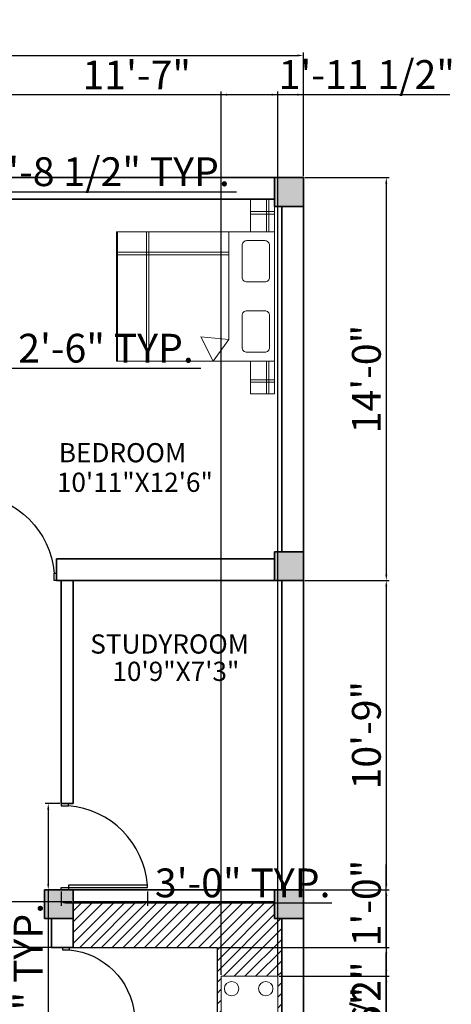
# Model space of a CAD drawing. Units: inches. Extents: x 2430 to 3058, y 1630 to 2396.
# Tile 4 of 4: x 2878 to 3058, y 1945 to 2356. Entities that reach past the tile are written whole.
import ezdxf

# ---------------------------------------------------------------- set-up
doc = ezdxf.new("R2010")
doc.units = ezdxf.units.IN
for name, color, linetype, lineweight in [('A-ANNO-DIMS', 7, 'Continuous', 18), ('A-AREA-IDEN', 131, 'Continuous', 18), ('A-COLS', 7, 'Continuous', 35), ('A-COLS-PATT', 1, 'Continuous', 13), ('A-DOOR', 40, 'Continuous', 25), ('A-FLOR-CASE', 7, 'Continuous', 25), ('A-FLOR-CASE-PATT', 131, 'Continuous', 13), ('A-WALL', 7, 'Continuous', 35)]:
    doc.layers.add(name, color=color, linetype=linetype, lineweight=lineweight)
doc.layers.add('A-EQPM', color=33, linetype='Continuous', lineweight=18, true_color=0xb0a07d)
doc.layers.add('A-FURN', color=33, linetype='Continuous', lineweight=18, true_color=0xb0a07d)
doc.styles.get("Standard").update_dxf_attribs({"font": 'arial.ttf'})
doc.dimstyles.new('ISO-25', dxfattribs={"dimtxt": 12, "dimasz": 2.5, "dimexe": 1.25, "dimexo": 0.625, "dimtad": 1, "dimdec": 0, "dimlunit": 3, "dimtxsty": 'Standard', "dimcen": 2.5, "dimadec": 0, "dimazin": 0, "dimtfac": 1, "dimtdec": 0, "dimtmove": 0, "dimatfit": 3, "dimfxl": 1, "dimarcsym": 0})

# ---------------------------------------------------------------- blocks, each defined once
blk = doc.blocks.new('*D1')
at = {"layer": 'A-ANNO-DIMS', "color": 0, "lineweight": -2, "transparency": 16777216}
for p, q in [((2636, 2290.5), (2636, 2342.06)), ((2638.5, 2340.81), (2993.5, 2340.81)), ((2996, 2290.5), (2996, 2342.06))]:
    blk.add_line(p, q, dxfattribs=at)
at = {"layer": 'A-ANNO-DIMS', "color": 0, "transparency": 16777216}
for points in [[(2638.5, 2341.22), (2638.5, 2340.39), (2636, 2340.81)], [(2993.5, 2341.22), (2993.5, 2340.39), (2996, 2340.81)]]:
    blk.add_solid(points, dxfattribs=at)
at = {"layer": 'Defpoints', "color": 0, "transparency": 16777216}
for p in [(2996, 2340.81), (2636, 2289.88), (2996, 2289.88)]:
    blk.add_point(p, dxfattribs=at)
at = {"layer": 'A-ANNO-DIMS', "color": 0, "transparency": 16777216, "insert": (2816, 2347.56), "char_height": 12, "attachment_point": 5}
blk.add_mtext("30'", dxfattribs=at)
blk = doc.blocks.new('BED-DOUBLE')
for p, q in [((0, 67.56), (0, 81.12)), ((0, 81.12), (10, 81.12)), ((2.41, 67.56), (2.41, 81.12)), ((3.41, 67.56), (3.41, 81.12)), ((10, 81.12), (10, 67.56)), ((10, 76.33), (0, 76.33)), ((10, 75.33), (0, 75.33)), ((19.07, 58.56), (25.57, 67.56)), ((25.57, 67.56), (30.72, 57.43)), ((52.45, 67.56), (52.45, 13.56)), ((53.45, 67.56), (53.45, 13.56)), ((65.45, 67.56), (65.45, 13.56)), ((19.07, 13.56), (19.07, 58.56)), ((30.72, 57.43), (19.07, 58.56)), ((19.07, 23.13), (66, 23.13)), ((19.07, 22.13), (66, 22.13)), ((0, 0), (0, 13.56)), ((2.41, 0), (2.41, 13.56)), ((3.41, 0), (3.41, 13.56)), ((10, 13.56), (10, 0)), ((10, 6.18), (0, 6.18)), ((10, 5.18), (0, 5.18)), ((0, 0), (10, 0))]:
    blk.add_line(p, q)
blk.add_lwpolyline([(0, 67.56), (66, 67.56), (66, 13.56), (0, 13.56)], close=True)
for points in [[(4.09, 63.78), (11.52, 63.78, -0.414214), (13.52, 61.78), (13.52, 48.53, -0.414214), (11.52, 46.53), (4.09, 46.53, -0.414214), (2.09, 48.53), (2.09, 61.78, -0.414214)], [(4.09, 34.52), (11.52, 34.52, -0.414214), (13.52, 32.52), (13.52, 19.27, -0.414214), (11.52, 17.27), (4.09, 17.27, -0.414214), (2.09, 19.27), (2.09, 32.52, -0.414214)]]:
    blk.add_lwpolyline(points, format="xyb", close=True)
blk = doc.blocks.new('DOOR-36')
for p, q in [((35, 36), (34, 36)), ((34, 36), (34, 3)), ((35, 0), (35, 36)), ((1, 3), (0, 3)), ((0, 0), (1, 0)), ((1, 0), (1, 3)), ((34, 3), (36, 3)), ((36, 0), (35, 0))]:
    blk.add_line(p, q)
blk.add_arc((36.88, 0.12), 36, 94.5954, 175.4046)
blk = doc.blocks.new('DOOR-30')
for p, q in [((0, 30), (0, 29)), ((0, 29), (30, 29)), ((3, 28), (3, 30)), ((30, 29), (30, 28)), ((30, 28), (3, 28)), ((0, 0), (0, 1)), ((0, 1), (3, 1)), ((3, 1), (3, 0))]:
    blk.add_line(p, q)
blk.add_arc((0.14, 30.86), 30, 275.4764, 354.5236)
blk = doc.blocks.new('COL-12x12-EDGE')
for p, q in [((12, 12), (0, 12)), ((0, 12), (0, 0)), ((0, 0), (12, 0))]:
    blk.add_line(p, q)
blk = doc.blocks.new('COL-12x12')
for p, q in [((12, 12), (0, 12)), ((0, 12), (0, 0)), ((12, 0), (12, 12)), ((0, 0), (12, 0))]:
    blk.add_line(p, q)
blk = doc.blocks.new('*D17')
at = {"layer": 'A-ANNO-DIMS', "color": 0, "lineweight": -2, "transparency": 16777216}
for p, q in [((2809.48, 2281.5), (2809.48, 2285.22)), ((2811.98, 2283.97), (2827.61, 2283.97)), ((2830.11, 2281.5), (2830.11, 2285.22)), ((2830.11, 2283.97), (2968.05, 2283.97))]:
    blk.add_line(p, q, dxfattribs=at)
at = {"layer": 'A-ANNO-DIMS', "color": 0, "transparency": 16777216}
for points in [[(2811.98, 2284.39), (2811.98, 2283.56), (2809.48, 2283.97)], [(2827.61, 2284.39), (2827.61, 2283.56), (2830.11, 2283.97)]]:
    blk.add_solid(points, dxfattribs=at)
at = {"layer": 'Defpoints', "color": 0, "transparency": 16777216}
for p in [(2830.11, 2283.97), (2809.48, 2280.88), (2830.11, 2280.88)]:
    blk.add_point(p, dxfattribs=at)
at = {"layer": 'A-ANNO-DIMS', "color": 0, "transparency": 16777216, "insert": (2900.33, 2290.8), "char_height": 12, "attachment_point": 5}
blk.add_mtext('WC 1\'-8 1/2" TYP.', dxfattribs=at)
blk = doc.blocks.new('*D19')
at = {"layer": 'A-ANNO-DIMS', "color": 0, "lineweight": -2, "transparency": 16777216}
for p, q in [((2894.37, 2028.88), (2888.35, 2028.88)), ((2889.6, 2026.38), (2889.6, 1995.38)), ((2894.37, 1992.88), (2888.35, 1992.88)), ((2889.6, 1992.88), (2889.6, 1861.63))]:
    blk.add_line(p, q, dxfattribs=at)
at = {"layer": 'A-ANNO-DIMS', "color": 0, "transparency": 16777216}
for points in [[(2889.18, 2026.38), (2890.01, 2026.38), (2889.6, 2028.88)], [(2889.18, 1995.38), (2890.01, 1995.38), (2889.6, 1992.88)]]:
    blk.add_solid(points, dxfattribs=at)
at = {"layer": 'Defpoints', "color": 0, "transparency": 16777216}
for p in [(2895, 2028.88), (2889.6, 1992.88), (2895, 1992.88)]:
    blk.add_point(p, dxfattribs=at)
at = {"layer": 'A-ANNO-DIMS', "color": 0, "transparency": 16777216, "insert": (2882.76, 1926), "char_height": 12, "attachment_point": 5, "rotation": 90}
blk.add_mtext('DOOR 3\'-0" TYP.', dxfattribs=at)
blk = doc.blocks.new('*D20')
at = {"layer": 'A-ANNO-DIMS', "color": 0, "lineweight": -2, "transparency": 16777216}
for p, q in [((2895, 1992.25), (2895, 1986.23)), ((2931, 1992.25), (2931, 1986.23)), ((2897.5, 1987.48), (2928.5, 1987.48)), ((2931, 1987.48), (3007.88, 1987.48))]:
    blk.add_line(p, q, dxfattribs=at)
at = {"layer": 'A-ANNO-DIMS', "color": 0, "transparency": 16777216}
for points in [[(2897.5, 1987.89), (2897.5, 1987.06), (2895, 1987.48)], [(2928.5, 1987.89), (2928.5, 1987.06), (2931, 1987.48)]]:
    blk.add_solid(points, dxfattribs=at)
at = {"layer": 'Defpoints', "color": 0, "transparency": 16777216}
for p in [(2895, 1992.88), (2931, 1992.88), (2931, 1987.48)]:
    blk.add_point(p, dxfattribs=at)
at = {"layer": 'A-ANNO-DIMS', "color": 0, "transparency": 16777216, "insert": (2970.69, 1994.23), "char_height": 12, "attachment_point": 5}
blk.add_mtext('3\'-0" TYP.', dxfattribs=at)
blk = doc.blocks.new('*D21')
at = {"layer": 'A-ANNO-DIMS', "color": 0, "lineweight": -2, "transparency": 16777216}
for p, q in [((2792, 2206.5), (2792, 2211.63)), ((2794.5, 2210.38), (2819.5, 2210.38)), ((2822, 2206.5), (2822, 2211.63)), ((2822, 2210.38), (2953.24, 2210.38))]:
    blk.add_line(p, q, dxfattribs=at)
at = {"layer": 'A-ANNO-DIMS', "color": 0, "transparency": 16777216}
for points in [[(2794.5, 2210.79), (2794.5, 2209.96), (2792, 2210.38)], [(2819.5, 2210.79), (2819.5, 2209.96), (2822, 2210.38)]]:
    blk.add_solid(points, dxfattribs=at)
at = {"layer": 'Defpoints', "color": 0, "transparency": 16777216}
for p in [(2822, 2210.38), (2792, 2205.88), (2822, 2205.88)]:
    blk.add_point(p, dxfattribs=at)
at = {"layer": 'A-ANNO-DIMS', "color": 0, "transparency": 16777216, "insert": (2888.87, 2217.21), "char_height": 12, "attachment_point": 5}
blk.add_mtext('DOOR 2\'-6" TYP.', dxfattribs=at)
blk = doc.blocks.new('*D29')
at = {"layer": 'A-ANNO-DIMS', "color": 0, "lineweight": -2, "transparency": 16777216}
for p, q in [((2857, 2281.5), (2857, 2325.73)), ((2859.5, 2324.48), (2993.5, 2324.48)), ((2996, 2290.5), (2996, 2325.73))]:
    blk.add_line(p, q, dxfattribs=at)
at = {"layer": 'A-ANNO-DIMS', "color": 0, "transparency": 16777216}
for points in [[(2859.5, 2324.89), (2859.5, 2324.06), (2857, 2324.48)], [(2993.5, 2324.89), (2993.5, 2324.06), (2996, 2324.48)]]:
    blk.add_solid(points, dxfattribs=at)
at = {"layer": 'Defpoints', "color": 0, "transparency": 16777216}
for p in [(2996, 2324.48), (2996, 2289.88), (2857, 2280.88)]:
    blk.add_point(p, dxfattribs=at)
at = {"layer": 'A-ANNO-DIMS', "color": 0, "transparency": 16777216, "insert": (2926.5, 2331.13), "char_height": 12, "attachment_point": 5}
blk.add_mtext('11\'-7"', dxfattribs=at)
blk = doc.blocks.new('*D30')
at = {"layer": 'A-ANNO-DIMS', "color": 0, "lineweight": -2, "transparency": 16777216}
for p, q in [((2996.62, 2289.88), (3031.85, 2289.88)), ((3030.6, 2287.38), (3030.6, 2124.38)), ((2996.62, 2121.88), (3031.85, 2121.88))]:
    blk.add_line(p, q, dxfattribs=at)
at = {"layer": 'A-ANNO-DIMS', "color": 0, "transparency": 16777216}
for points in [[(3030.18, 2287.38), (3031.01, 2287.38), (3030.6, 2289.88)], [(3030.18, 2124.38), (3031.01, 2124.38), (3030.6, 2121.88)]]:
    blk.add_solid(points, dxfattribs=at)
at = {"layer": 'Defpoints', "color": 0, "transparency": 16777216}
for p in [(2996, 2289.88), (2996, 2121.88), (3030.6, 2121.88)]:
    blk.add_point(p, dxfattribs=at)
at = {"layer": 'A-ANNO-DIMS', "color": 0, "transparency": 16777216, "insert": (3023.84, 2205.88), "char_height": 12, "attachment_point": 5, "rotation": 90}
blk.add_mtext('14\'-0"', dxfattribs=at)
blk = doc.blocks.new('*D31')
at = {"layer": 'A-ANNO-DIMS', "color": 0, "lineweight": -2, "transparency": 16777216}
for p, q in [((2996.62, 2121.88), (3031.85, 2121.88)), ((3030.6, 2119.38), (3030.6, 1995.38)), ((2996.62, 1992.88), (3031.85, 1992.88))]:
    blk.add_line(p, q, dxfattribs=at)
at = {"layer": 'A-ANNO-DIMS', "color": 0, "transparency": 16777216}
for points in [[(3030.18, 2119.38), (3031.01, 2119.38), (3030.6, 2121.88)], [(3030.18, 1995.38), (3031.01, 1995.38), (3030.6, 1992.88)]]:
    blk.add_solid(points, dxfattribs=at)
at = {"layer": 'Defpoints', "color": 0, "transparency": 16777216}
for p in [(2996, 2121.88), (2996, 1992.88), (3030.6, 1992.88)]:
    blk.add_point(p, dxfattribs=at)
at = {"layer": 'A-ANNO-DIMS', "color": 0, "transparency": 16777216, "insert": (3023.84, 2057.38), "char_height": 12, "attachment_point": 5, "rotation": 90}
blk.add_mtext('10\'-9"', dxfattribs=at)
blk = doc.blocks.new('*D32')
at = {"layer": 'A-ANNO-DIMS', "color": 0, "lineweight": -2, "transparency": 16777216}
for p, q in [((2996.62, 1992.88), (3031.85, 1992.88)), ((3030.6, 1990.38), (3030.6, 1869.38)), ((2987.62, 1866.88), (3031.85, 1866.88))]:
    blk.add_line(p, q, dxfattribs=at)
at = {"layer": 'A-ANNO-DIMS', "color": 0, "transparency": 16777216}
for points in [[(3030.18, 1990.38), (3031.01, 1990.38), (3030.6, 1992.88)], [(3030.18, 1869.38), (3031.01, 1869.38), (3030.6, 1866.88)]]:
    blk.add_solid(points, dxfattribs=at)
at = {"layer": 'Defpoints', "color": 0, "transparency": 16777216}
for p in [(2996, 1992.88), (2987, 1866.88), (3030.6, 1866.88)]:
    blk.add_point(p, dxfattribs=at)
at = {"layer": 'A-ANNO-DIMS', "color": 0, "transparency": 16777216, "insert": (3023.84, 1929.88), "char_height": 12, "attachment_point": 5, "rotation": 90}
blk.add_mtext('10\'-6"', dxfattribs=at)
blk = doc.blocks.new('*D49')
at = {"layer": 'A-ANNO-DIMS', "color": 0, "lineweight": -2, "transparency": 16777216}
for p, q in [((2840.99, 2130.25), (2840.99, 1630.03)), ((2852, 2130.25), (2852, 1630.03)), ((2843.49, 1631.28), (2849.5, 1631.28)), ((2852, 1631.28), (2896.97, 1631.28))]:
    blk.add_line(p, q, dxfattribs=at)
at = {"layer": 'A-ANNO-DIMS', "color": 0, "transparency": 16777216}
for points in [[(2843.49, 1631.69), (2843.49, 1630.86), (2840.99, 1631.28)], [(2849.5, 1631.69), (2849.5, 1630.86), (2852, 1631.28)]]:
    blk.add_solid(points, dxfattribs=at)
at = {"layer": 'Defpoints', "color": 0, "transparency": 16777216}
for p in [(2840.99, 2130.88), (2852, 2130.88), (2852, 1631.28)]:
    blk.add_point(p, dxfattribs=at)
at = {"layer": 'A-ANNO-DIMS', "color": 0, "transparency": 16777216, "insert": (2875.73, 1638.03), "char_height": 12, "attachment_point": 5}
blk.add_mtext('0\'-11"', dxfattribs=at)
blk = doc.blocks.new('*D51')
at = {"layer": 'A-ANNO-DIMS', "color": 0, "lineweight": -2, "transparency": 16777216}
for p, q in [((2601.4, 1987.88), (2601.4, 2022.4)), ((2899.37, 1987.88), (2600.15, 1987.88)), ((2601.4, 1971.38), (2601.4, 1985.38)), ((2899.37, 1968.88), (2600.15, 1968.88))]:
    blk.add_line(p, q, dxfattribs=at)
at = {"layer": 'A-ANNO-DIMS', "color": 0, "transparency": 16777216}
for points in [[(2600.98, 1985.38), (2601.81, 1985.38), (2601.4, 1987.88)], [(2600.98, 1971.38), (2601.81, 1971.38), (2601.4, 1968.88)]]:
    blk.add_solid(points, dxfattribs=at)
at = {"layer": 'Defpoints', "color": 0, "transparency": 16777216}
for p in [(2601.4, 1987.88), (2900, 1987.88), (2900, 1968.88)]:
    blk.add_point(p, dxfattribs=at)
at = {"layer": 'A-ANNO-DIMS', "color": 0, "transparency": 16777216, "insert": (2594.75, 2006.39), "char_height": 12, "attachment_point": 5, "rotation": 90}
blk.add_mtext('1\'-7"', dxfattribs=at)
blk = doc.blocks.new('*D52')
at = {"layer": 'A-ANNO-DIMS', "color": 0, "lineweight": -2, "transparency": 16777216}
for p, q in [((2961.68, 1957.48), (2961.68, 2325.73)), ((2964.18, 2324.48), (2982.8, 2324.48)), ((2985.3, 1957.48), (2985.3, 2325.73)), ((2985.3, 2324.48), (3057.1, 2324.48))]:
    blk.add_line(p, q, dxfattribs=at)
at = {"layer": 'A-ANNO-DIMS', "color": 0, "transparency": 16777216}
for points in [[(2964.18, 2324.89), (2964.18, 2324.06), (2961.68, 2324.48)], [(2982.8, 2324.89), (2982.8, 2324.06), (2985.3, 2324.48)]]:
    blk.add_solid(points, dxfattribs=at)
at = {"layer": 'Defpoints', "color": 0, "transparency": 16777216}
for p in [(2985.3, 2324.48), (2961.68, 1956.85), (2985.3, 1956.85)]:
    blk.add_point(p, dxfattribs=at)
at = {"layer": 'A-ANNO-DIMS', "color": 0, "transparency": 16777216, "insert": (3022.45, 2331.31), "char_height": 12, "attachment_point": 5}
blk.add_mtext('1\'-11 1/2"', dxfattribs=at)
blk = doc.blocks.new('*D53')
at = {"layer": 'A-ANNO-DIMS', "color": 0, "lineweight": -2, "transparency": 16777216}
for p, q in [((2985.92, 1956.85), (3031.85, 1956.85)), ((3030.6, 1954.35), (3030.6, 1929.42)), ((2985.92, 1926.92), (3031.85, 1926.92)), ((3030.6, 1926.92), (3030.6, 1891.07))]:
    blk.add_line(p, q, dxfattribs=at)
at = {"layer": 'A-ANNO-DIMS', "color": 0, "transparency": 16777216}
for points in [[(3030.18, 1954.35), (3031.01, 1954.35), (3030.6, 1956.85)], [(3030.18, 1929.42), (3031.01, 1929.42), (3030.6, 1926.92)]]:
    blk.add_solid(points, dxfattribs=at)
at = {"layer": 'Defpoints', "color": 0, "transparency": 16777216}
for p in [(2985.3, 1956.85), (2985.3, 1926.92), (3030.6, 1926.92)]:
    blk.add_point(p, dxfattribs=at)
at = {"layer": 'A-ANNO-DIMS', "color": 0, "transparency": 16777216, "insert": (3023.84, 1907.75), "char_height": 12, "attachment_point": 5, "rotation": 90}
blk.add_mtext('2\'-6"', dxfattribs=at)
blk = doc.blocks.new('*D55')
at = {"layer": 'A-ANNO-DIMS', "color": 0, "lineweight": -2, "transparency": 16777216}
for p, q in [((3030.6, 1898.4), (3030.6, 1960.88)), ((2984.38, 1898.4), (3031.85, 1898.4)), ((3030.6, 1879.56), (3030.6, 1895.9)), ((2984.38, 1877.06), (3031.85, 1877.06))]:
    blk.add_line(p, q, dxfattribs=at)
at = {"layer": 'A-ANNO-DIMS', "color": 0, "transparency": 16777216}
for points in [[(3030.18, 1895.9), (3031.01, 1895.9), (3030.6, 1898.4)], [(3030.18, 1879.56), (3031.01, 1879.56), (3030.6, 1877.06)]]:
    blk.add_solid(points, dxfattribs=at)
at = {"layer": 'Defpoints', "color": 0, "transparency": 16777216}
for p in [(2983.75, 1898.4), (3030.6, 1898.4), (2983.75, 1877.06)]:
    blk.add_point(p, dxfattribs=at)
at = {"layer": 'A-ANNO-DIMS', "color": 0, "transparency": 16777216, "insert": (3023.77, 1930.89), "char_height": 12, "attachment_point": 5, "rotation": 90}
blk.add_mtext('1\'-9 1/2"', dxfattribs=at)
blk = doc.blocks.new('*D56')
at = {"layer": 'A-ANNO-DIMS', "color": 0, "lineweight": -2, "transparency": 16777216}
for p, q in [((3030.6, 1968.88), (3030.6, 2003.4)), ((2960.62, 1968.88), (3031.85, 1968.88)), ((3030.6, 1959.35), (3030.6, 1966.38)), ((2985.92, 1956.85), (3031.85, 1956.85))]:
    blk.add_line(p, q, dxfattribs=at)
at = {"layer": 'A-ANNO-DIMS', "color": 0, "transparency": 16777216}
for points in [[(3030.18, 1966.38), (3031.01, 1966.38), (3030.6, 1968.88)], [(3030.18, 1959.35), (3031.01, 1959.35), (3030.6, 1956.85)]]:
    blk.add_solid(points, dxfattribs=at)
at = {"layer": 'Defpoints', "color": 0, "transparency": 16777216}
for p in [(2960, 1968.88), (3030.6, 1968.88), (2985.3, 1956.85)]:
    blk.add_point(p, dxfattribs=at)
at = {"layer": 'A-ANNO-DIMS', "color": 0, "transparency": 16777216, "insert": (3023.84, 1987.39), "char_height": 12, "attachment_point": 5, "rotation": 90}
blk.add_mtext('1\'-0"', dxfattribs=at)

msp = doc.modelspace()

# ---------------------------------------------------------------- hatches: boundary and pattern name
at = {"layer": 'A-COLS-PATT'}
h = msp.add_hatch(color=256, dxfattribs=at)
h.dxf.hatch_style = 1
h.paths.add_polyline_path([(2996, 2289.88), (2984, 2289.88), (2984, 2277.88), (2996, 2277.88)])
h = msp.add_hatch(color=256, dxfattribs=at)
h.dxf.hatch_style = 1
h.paths.add_polyline_path([(2996, 2133.88), (2984, 2133.88), (2984, 2121.88), (2996, 2121.88)])
h = msp.add_hatch(color=256, dxfattribs=at)
h.dxf.hatch_style = 1
h.paths.add_polyline_path([(2900, 1992.88), (2891, 1992.88), (2888, 1992.88), (2888, 1980.88), (2900, 1980.88)])
h = msp.add_hatch(color=256, dxfattribs=at)
h.dxf.hatch_style = 1
h.paths.add_polyline_path([(2996, 1992.88), (2984, 1992.88), (2984, 1980.88), (2996, 1980.88)])
at = {"layer": 'A-FLOR-CASE-PATT'}
h = msp.add_hatch(dxfattribs=at)
h.set_pattern_fill('ANSI31', color=256)
h.paths.add_polyline_path([(2987, 1980.88), (2984, 1980.88), (2984, 1987.88), (2900, 1987.88), (2900, 1968.88), (2960, 1968.88), (2960, 1871.88), (2987, 1871.88)])
h.paths.add_polyline_path([(2961.68, 1956.85), (2985.3, 1956.85), (2985.3, 1926.92), (2961.68, 1926.92)], flags=16)
h.paths.add_polyline_path([(2969.08, 1951.68, -1), (2963.08, 1951.68, -1)], flags=0)
h.paths.add_polyline_path([(2963.83, 1944.18), (2983.44, 1944.18), (2983.44, 1939.79), (2963.83, 1939.79)], flags=0)
h.paths.add_polyline_path([(2983.32, 1951.68, -1), (2977.32, 1951.68, -1)], flags=0)
h.paths.add_polyline_path([(2969.08, 1932.19, -1), (2963.08, 1932.19, -1)], flags=0)
h.paths.add_polyline_path([(2983.32, 1932.19, -1), (2977.32, 1932.19, -1)], flags=0)
h.paths.add_polyline_path([(2962.55, 1898.4), (2983.75, 1898.4), (2983.75, 1877.06), (2962.55, 1877.06)], flags=16)
h.paths.add_polyline_path([(2974.72, 1887.73, -1), (2971.58, 1887.73, -1)], flags=0)

# ---------------------------------------------------------------- linework, layer by layer
at = {"layer": 'A-COLS'}
for p, q in [((2891, 1992.88), (2888, 1992.88)), ((2888, 1992.88), (2888, 1980.88)), ((2888, 1980.88), (2900, 1980.88))]:
    msp.add_line(p, q, dxfattribs=at)
at = {"layer": 'A-EQPM'}
msp.add_lwpolyline([(2961.68, 1956.85), (2985.3, 1956.85), (2985.3, 1926.92), (2961.68, 1926.92)], close=True, dxfattribs=at)
for centre in [(2966.08, 1951.68), (2980.32, 1951.68)]:
    msp.add_circle(centre, 3, dxfattribs=at)
at = {"layer": 'A-FLOR-CASE'}
for p, q in [((2900, 1968.88), (2960, 1968.88)), ((2960, 1968.88), (2960, 1871.88))]:
    msp.add_line(p, q, dxfattribs=at)
at = {"layer": 'A-WALL'}
for p, q in [((2804, 2280.88), (2984, 2280.88)), ((2987, 2277.88), (2987, 2133.88)), ((2893, 2130.88), (2893, 2121.88)), ((2893, 2130.88), (2984, 2130.88)), ((2893, 2121.88), (2987, 2121.88)), ((2895, 2121.88), (2895, 2028.88)), ((2900, 2121.88), (2900, 2028.88)), ((2987, 2121.88), (2987, 1992.88)), ((2895, 2028.88), (2900, 2028.88)), ((2891, 1992.88), (2987, 1992.88)), ((2900, 1992.88), (2900, 1987.88)), ((2900, 1992.88), (2900, 1968.88)), ((2900, 1987.88), (2984, 1987.88)), ((2891, 1980.88), (2891, 1968.88)), ((2987, 1980.88), (2987, 1845.6)), ((2891, 1968.88), (2900, 1968.88))]:
    msp.add_line(p, q, dxfattribs=at)
msp.add_lwpolyline([(2636, 2289.88), (2996, 2289.88), (2996, 1689.88), (2636, 1689.88)], close=True, dxfattribs=at)

# ---------------------------------------------------------------- block references
at = {"layer": 'A-COLS'}
for name, p in [('COL-12x12-EDGE', (2984, 2277.88)), ('COL-12x12', (2984, 2121.88)), ('COL-12x12-EDGE', (2984, 1980.88))]:
    msp.add_blockref(name, p, dxfattribs=at)
at = {"layer": 'A-DOOR', "extrusion": (0, 0, -1), "zscale": -1}
msp.add_blockref('DOOR-36', (-2893, 2121.88), dxfattribs=at)
at = {"layer": 'A-DOOR', "rotation": 270.0000000000037}
msp.add_blockref('DOOR-36', (2895, 2028.88), dxfattribs=at)
at = {"layer": 'A-DOOR', "extrusion": (0, 0, -1), "zscale": -1, "rotation": 180}
msp.add_blockref('DOOR-30', (-2895.5, 1968.88), dxfattribs=at)
at = {"layer": 'A-FURN', "rotation": 180}
msp.add_blockref('BED-DOUBLE', (2984, 2280.88), dxfattribs=at)

# ---------------------------------------------------------------- texts
at = {"layer": 'A-AREA-IDEN'}
for tag, p in [('BEDROOM', (2894.02, 2171.17)), ('10\'11"X12\'6"', (2893.2, 2158.84)), ('STUDYROOM', (2907.12, 2091.4)), ('10\'9"X7\'3"', (2916.35, 2080))]:
    msp.add_attdef(tag, p, '', height=8, dxfattribs=at)

# ---------------------------------------------------------------- dimensions: what is measured, and where the dimension line sits
at = {"layer": 'A-ANNO-DIMS'}
for base, p1, p2, override, picture, middle in [((2996, 2340.81), (2636, 2289.88), (2996, 2289.88), {"dimclrd": 0, "dimclre": 0, "dimclrt": 0}, '*D1', (2816, 2347.56)), ((2985.3, 2324.48), (2961.68, 1956.85), (2985.3, 1956.85), {"dimdec": 1, "dimlfac": 1, "dimrnd": 0, "dimzin": 1, "dimdsep": 46, "dimlunit": 4, "dimfrac": 2}, '*D52', (3022.45, 2331.31)), ((2996, 2324.48), (2857, 2280.88), (2996, 2289.88), {"dimdec": 1, "dimlfac": 1, "dimrnd": 0, "dimzin": 1, "dimdsep": 46, "dimlunit": 4, "dimfrac": 2}, '*D29', (2926.5, 2331.13)), ((2852, 1631.28), (2840.99, 2130.88), (2852, 2130.88), {"dimdec": 1, "dimlfac": 1, "dimrnd": 0, "dimzin": 1, "dimdsep": 46, "dimlunit": 4, "dimfrac": 2}, '*D49', (2875.73, 1638.03))]:
    dim = msp.add_linear_dim(base=base, p1=p1, p2=p2, dimstyle='ISO-25', override=override, dxfattribs=at)
    dim.commit()
    dim.dimension.update_dxf_attribs({"geometry": picture, "text_midpoint": middle})
for base, p1, p2, text, picture, middle in [((2830.11, 2283.97), (2809.48, 2280.88), (2830.11, 2280.88), 'WC <> TYP.', '*D17', (2900.33, 2290.8)), ((2822, 2210.38), (2792, 2205.88), (2822, 2205.88), 'DOOR <> TYP.', '*D21', (2888.87, 2217.21))]:
    dim = msp.add_linear_dim(base=base, p1=p1, p2=p2, text=text, dimstyle='ISO-25', override={"dimdec": 1, "dimlfac": 1, "dimrnd": 0, "dimzin": 1, "dimdsep": 46, "dimlunit": 4, "dimfrac": 2}, dxfattribs=at)
    dim.commit()
    dim.dimension.update_dxf_attribs({"geometry": picture, "text_midpoint": middle})
for base, p1, p2, picture, middle in [((3030.6, 2121.88), (2996, 2289.88), (2996, 2121.88), '*D30', (3023.84, 2205.88)), ((3030.6, 1992.88), (2996, 2121.88), (2996, 1992.88), '*D31', (3023.84, 2057.38)), ((2601.4, 1987.88), (2900, 1968.88), (2900, 1987.88), '*D51', (2594.75, 2006.39)), ((3030.6, 1968.88), (2985.3, 1956.85), (2960, 1968.88), '*D56', (3023.84, 1987.39)), ((3030.6, 1866.88), (2996, 1992.88), (2987, 1866.88), '*D32', (3023.84, 1929.88)), ((3030.6, 1898.4), (2983.75, 1877.06), (2983.75, 1898.4), '*D55', (3023.77, 1930.89)), ((3030.6, 1926.92), (2985.3, 1956.85), (2985.3, 1926.92), '*D53', (3023.84, 1907.75))]:
    dim = msp.add_linear_dim(base=base, p1=p1, p2=p2, angle=90, dimstyle='ISO-25', override={"dimdec": 1, "dimlfac": 1, "dimrnd": 0, "dimzin": 1, "dimdsep": 46, "dimlunit": 4, "dimfrac": 2}, dxfattribs=at)
    dim.commit()
    dim.dimension.update_dxf_attribs({"geometry": picture, "text_midpoint": middle})
for base, p1, p2, angle, text, picture, middle in [((2889.6, 1992.88), (2895, 2028.88), (2895, 1992.88), 270, 'DOOR <> TYP.', '*D19', (2882.76, 1926)), ((2931, 1987.48), (2895, 1992.88), (2931, 1992.88), 0, '<> TYP.', '*D20', (2970.69, 1994.23))]:
    dim = msp.add_linear_dim(base=base, p1=p1, p2=p2, angle=angle, text=text, dimstyle='ISO-25', override={"dimdec": 1, "dimlfac": 1, "dimrnd": 0, "dimzin": 1, "dimdsep": 46, "dimlunit": 4, "dimfrac": 2}, dxfattribs=at)
    dim.commit()
    dim.dimension.update_dxf_attribs({"geometry": picture, "text_midpoint": middle})

doc.saveas('drawing.dxf')
